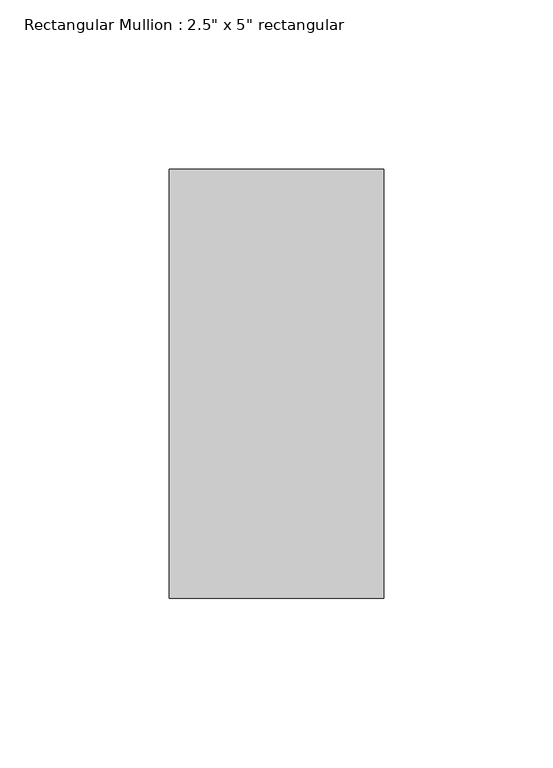
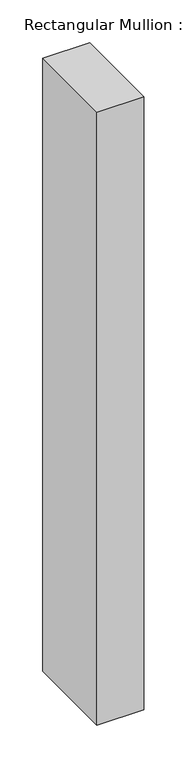
"""IFC4 building model written with IfcOpenShell, lengths in millimetres: member geometry."""

from ifc_helpers import new_model, si_unit, frame, origin, place, context, project, spatial, polyline, outline, extrude, source, transform, mapped, element, save


def member_99b0d556(model_context):
    return source(origin(), model_context, "Body", "SweptSolid", [
        extrude(outline(polyline([(0.0, 63.5), (0.0, -63.5), (-63.5, -63.5), (-63.5, 63.5), (0.0, 63.5)])), frame((0.0, 0.0, -876.3), z_axis=(0.0, 0.0, 1.0), x_axis=(1.0, 0.0, 0.0)), (0.0, 0.0, 1.0), 876.3),
    ])


if __name__ == "__main__":
    model = new_model("IFC4")
    model_context = context("Model", 3, world=origin())
    ifc_project = project(units=[si_unit("LENGTHUNIT", "METRE", prefix="MILLI")], contexts=[model_context])
    site = spatial("IfcSite", under=ifc_project)
    building = spatial("IfcBuilding", under=site)
    placement = place(None, origin())
    member_shape = member_99b0d556(model_context)
    element("IfcMember", 1, ObjectType="Rectangular Mullion : 2.5\" x 5\" rectangular", at=placement, inside=building, context=model_context, shape_type="MappedRepresentation", body=[
        mapped(member_shape, transform((0.0, 0.0, 0.0), x_axis=(1.0, 0.0, 0.0), y_axis=(0.0, 1.0, 0.0), z_axis=(0.0, 0.0, 1.0))),
    ])
    save(model, "model.ifc")

# Revit data of these elements
# Type "Rectangular Mullion : 2.5\" x 5\" rectangular"
#   built-in parameter 1007304 = 0.416667 (stored number, unit not read)
#   built-in parameter 1007301 = 0.104167 (stored number, unit not read)
#   built-in parameter 1007300 = 0.104167 (stored number, unit not read)
# Element 1 (IfcMember, "Rectangular Mullion : 2.5\" x 5\" rectangular")
#   Materials on its faces: "Aluminum"
# Materials
#   "Aluminum": class "Metal", colour RGB 247 247 247, transparency 0, Description = "Aluminum 6061", Cost = 0
